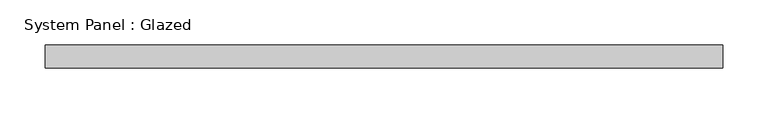
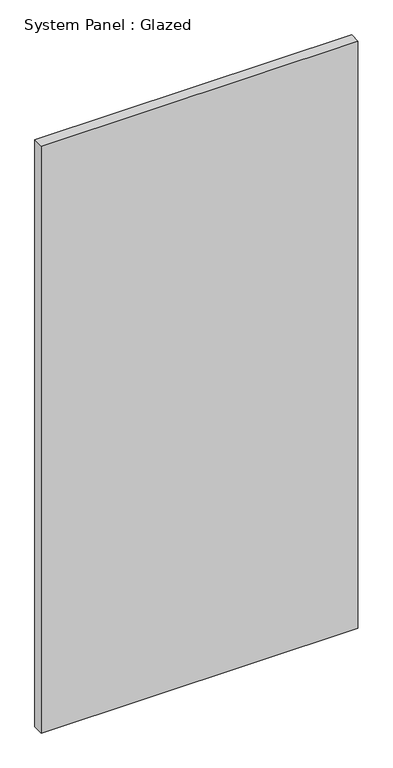
"""IFC4 building model written with IfcOpenShell, lengths in millimetres: plate geometry, System Panel : Glazed."""

from ifc_helpers import new_model, si_unit, origin, origin_with_axes, place, context, project, spatial, polyline, outline, extrude, source, transform, mapped, element, save


def system_panel_glazed_230baa0e(model_context):
    return source(origin(), model_context, "Body", "SweptSolid", [
        extrude(outline(polyline([(372.7688551, 19.05), (-372.7688551, 19.05), (-372.7688551, 44.45), (372.7688551, 44.45), (372.7688551, 19.05)])), origin_with_axes(), (0.0, 0.0, 1.0), 1460.5291864),
    ])


if __name__ == "__main__":
    model = new_model("IFC4")
    model_context = context("Model", 3, world=origin())
    ifc_project = project(units=[si_unit("LENGTHUNIT", "METRE", prefix="MILLI")], contexts=[model_context])
    site = spatial("IfcSite", under=ifc_project)
    building = spatial("IfcBuilding", under=site)
    placement = place(None, origin())
    system_panel_glazed_shape = system_panel_glazed_230baa0e(model_context)
    element("IfcPlate", 1, ObjectType="System Panel : Glazed", at=placement, inside=building, context=model_context, shape_type="MappedRepresentation", body=[
        mapped(system_panel_glazed_shape, transform((0.0, 0.0, 0.0), x_axis=(1.0, 0.0, 0.0), y_axis=(0.0, 1.0, 0.0), z_axis=(0.0, 0.0, 1.0))),
    ])
    save(model, "model.ifc")

# Revit data of these elements
# Type "System Panel : Glazed"
#   Construction Type Id = "GSP4R"
#   Analytic Construction = "1/8 in Pilkington single glazing"
#   Visual Light Transmittance = 0.9
#   Solar Heat Gain Coefficient = 0.86
#   Heat Transfer Coefficient (U) = 1.18115 BTU/(h·ft²·°F)
#   Define Thermal Properties by = 1
# Element 1 (IfcPlate, "System Panel : Glazed")
#   Materials on its faces: "Glass"
# Materials
#   "Glass": class "Glass", colour RGB 0 128 192, transparency 0.75, Description = "Soda Lime Glass", Cost = 0
